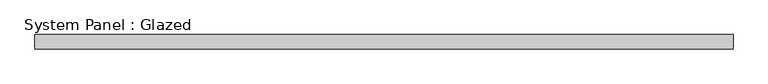
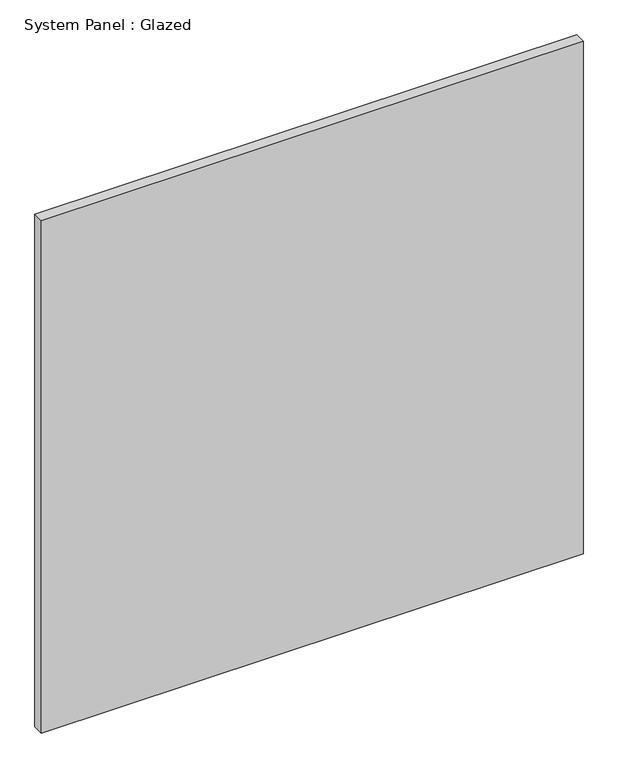
"""IFC4 building model written with IfcOpenShell, lengths in millimetres: plate geometry, System Panel : Glazed."""

from ifc_helpers import new_model, si_unit, origin, origin_with_axes, place, context, project, spatial, polyline, outline, extrude, source, transform, mapped, element, save


def system_panel_glazed_84cf4e26(model_context):
    return source(origin(), model_context, "Body", "SweptSolid", [
        extrude(outline(polyline([(609.6, 19.05), (-609.6, 19.05), (-609.6, 44.45), (609.6, 44.45), (609.6, 19.05)])), origin_with_axes(), (0.0, 0.0, 1.0), 1219.2),
    ])


if __name__ == "__main__":
    model = new_model("IFC4")
    model_context = context("Model", 3, world=origin())
    ifc_project = project(units=[si_unit("LENGTHUNIT", "METRE", prefix="MILLI")], contexts=[model_context])
    site = spatial("IfcSite", under=ifc_project)
    building = spatial("IfcBuilding", under=site)
    placement = place(None, origin())
    system_panel_glazed_shape = system_panel_glazed_84cf4e26(model_context)
    element("IfcPlate", 1, ObjectType="System Panel : Glazed", at=placement, inside=building, context=model_context, shape_type="MappedRepresentation", body=[
        mapped(system_panel_glazed_shape, transform((0.0, 0.0, 0.0), x_axis=(1.0, 0.0, 0.0), y_axis=(0.0, 1.0, 0.0), z_axis=(0.0, 0.0, 1.0))),
    ])
    save(model, "model.ifc")

# Revit data of these elements
# Type "System Panel : Glazed"
#   Construction Type Id = "GSP4R"
#   Analytic Construction = "1/8 in Pilkington single glazing"
#   Visual Light Transmittance = 0.9
#   Solar Heat Gain Coefficient = 0.86
#   Heat Transfer Coefficient (U) = 1.18115 BTU/(h·ft²·°F)
# Element 1 (IfcPlate, "System Panel : Glazed")
#   Materials on its faces: "Glass"
# Materials
#   "Glass": class "Glass", colour RGB 0 128 192, transparency 0.75, Description = "Soda Lime Glass", Cost = 0
